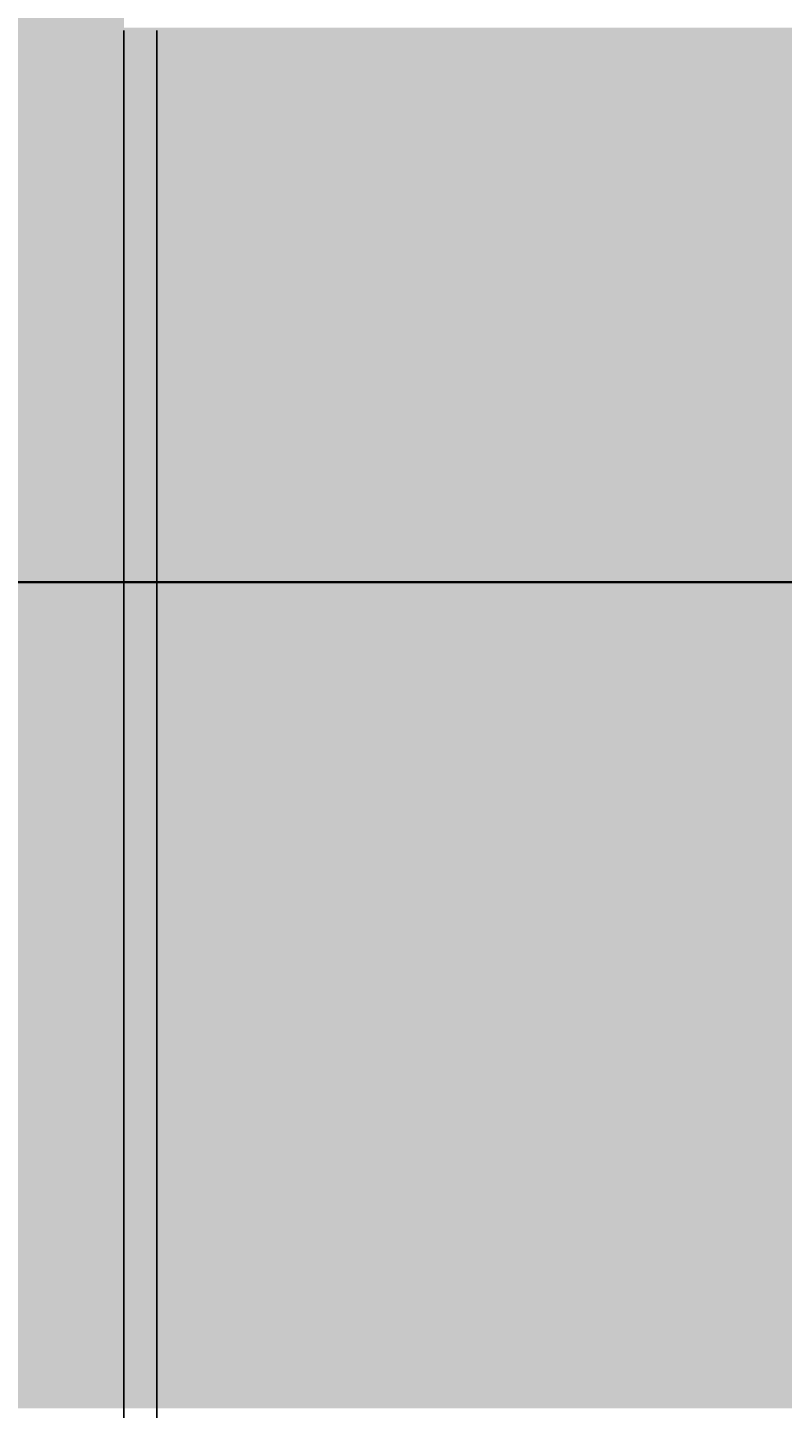
# Model space of a CAD drawing. Units: feet. Extents: x 2695 to 2912, y 795 to 1139.
# Tile 29 of 83: x 2808 to 2825, y 906 to 937. Entities that reach past the tile are written whole.
import ezdxf

# ---------------------------------------------------------------- set-up
doc = ezdxf.new("R2010")
doc.units = ezdxf.units.FT
for name, color, linetype, lineweight in [('A-ANNO-DIMS', 2, 'Continuous', 18), ('A-ELEV', 7, 'Continuous', 35), ('A-ELEV-PATT', 252, 'Continuous', 13)]:
    doc.layers.add(name, color=color, linetype=linetype, lineweight=lineweight)
doc.styles.get("Standard").update_dxf_attribs({"font": 'arial.ttf'})
doc.dimstyles.get("Standard").update_dxf_attribs({"dimtxt": 0.18, "dimasz": 0.18, "dimexe": 0.18, "dimexo": 0.0625, "dimgap": 0.09, "dimtad": 0, "dimtih": 1, "dimtoh": 1, "dimdec": 1, "dimzin": 0, "dimdsep": 46, "dimlunit": 3, "dimtxsty": 'Standard', "dimcen": 0.09, "dimadec": 0, "dimazin": 0, "dimtfac": 1, "dimtdec": 1, "dimtofl": 0, "dimtmove": 0, "dimatfit": 3, "dimfxl": 1, "dimtolj": 1, "dimtzin": 0, "dimarcsym": 0})

# ---------------------------------------------------------------- blocks, each defined once
blk = doc.blocks.new('*D14')
at = {"layer": 'A-ANNO-DIMS', "color": 0, "lineweight": -2, "transparency": 16777216}
for p, q in [((2838.439, 905.514), (2911.424, 905.514)), ((2911.244, 905.334), (2911.244, 890.368)), ((2911.244, 875.037), (2911.244, 890.004)), ((2758.214, 874.857), (2911.424, 874.857))]:
    blk.add_line(p, q, dxfattribs=at)
at = {"layer": 'A-ANNO-DIMS', "color": 0, "transparency": 16777216}
for points in [[(2911.214, 905.334), (2911.274, 905.334), (2911.244, 905.514)], [(2911.214, 875.037), (2911.274, 875.037), (2911.244, 874.857)]]:
    blk.add_solid(points, dxfattribs=at)
at = {"layer": 'Defpoints', "color": 0, "transparency": 16777216}
for p in [(2838.377, 905.514), (2911.244, 905.514), (2758.151, 874.857)]:
    blk.add_point(p, dxfattribs=at)
at = {"layer": 'A-ANNO-DIMS', "color": 0, "transparency": 16777216, "insert": (2911.244, 890.186), "char_height": 0.18, "attachment_point": 5}
blk.add_mtext('\\A1;30.66', dxfattribs=at)
blk = doc.blocks.new('*D52')
at = {"layer": 'A-ANNO-DIMS', "color": 0, "lineweight": -2, "transparency": 16777216}
for p, q in [((2810.041, 936.868), (2810.041, 794.976)), ((2810.789, 936.868), (2810.789, 794.976)), ((2809.861, 795.156), (2809.681, 795.156)), ((2810.969, 795.156), (2811.149, 795.156))]:
    blk.add_line(p, q, dxfattribs=at)
at = {"layer": 'A-ANNO-DIMS', "color": 0, "transparency": 16777216}
for points in [[(2809.861, 795.186), (2809.861, 795.126), (2810.041, 795.156)], [(2810.969, 795.186), (2810.969, 795.126), (2810.789, 795.156)]]:
    blk.add_solid(points, dxfattribs=at)
at = {"layer": 'Defpoints', "color": 0, "transparency": 16777216}
for p in [(2810.041, 936.931), (2810.789, 936.931), (2810.789, 795.156)]:
    blk.add_point(p, dxfattribs=at)
at = {"layer": 'A-ANNO-DIMS', "color": 0, "transparency": 16777216, "insert": (2810.415, 795.156), "char_height": 0.18, "attachment_point": 5}
blk.add_mtext('\\A1;0.75', dxfattribs=at)

msp = doc.modelspace()

# ---------------------------------------------------------------- hatches: boundary and pattern name
at = {"layer": 'A-ELEV-PATT'}
h = msp.add_hatch(color=256, dxfattribs=at)
h.set_gradient(color1=(255, 255, 255), tint=1)
h.paths.add_polyline_path([(2770.6361, 1122.9306), (2710.6361, 1122.9306), (2710.6361, 1118.4096), (2770.6361, 1118.4096)])
h.paths.add_polyline_path([(2890.6361, 1107.8588), (2770.6361, 1107.8588), (2770.6361, 1103.3378), (2890.6361, 1103.3378)])
h.paths.add_polyline_path([(2890.6361, 1062.9306), (2710.6361, 1062.9306), (2710.6361, 1056.9306), (2710.6361, 936.9306), (2710.6361, 924.3105), (2716.5358, 924.3105), (2890.6361, 924.3105), (2890.6361, 936.9306), (2715.8852, 936.9306), (2715.8852, 1050.3105), (2890.6361, 1050.3105)])
h.paths.add_polyline_path([(2716.5358, 924.3105), (2710.6361, 924.3105), (2710.6361, 810.9306), (2716.5358, 810.9306)])
h = msp.add_hatch(color=256, dxfattribs=at)
h.set_gradient(color1=(147, 149, 152), color2=(147, 149, 152), tint=1)
h.paths.add_polyline_path([(2770.6361, 1118.4096), (2710.6361, 1118.4096), (2710.6361, 1062.9306), (2770.6361, 1062.9306)])
h.paths.add_polyline_path([(2890.6361, 1103.3378), (2770.6361, 1103.3378), (2770.6361, 1062.9306), (2890.6361, 1062.9306)])
h.paths.add_polyline_path([(2730.7081, 1048.1052), (2755.1125, 1048.1052), (2755.1125, 936.9306), (2770.6361, 936.9306), (2770.6361, 1050.3105), (2715.8852, 1050.3105), (2715.8852, 936.9306), (2730.7081, 936.9306)])
h.paths.add_polyline_path([(2890.6361, 1050.3105), (2770.6361, 1050.3105), (2770.6361, 971.9673), (2778.0341, 971.9673), (2778.0341, 1020.8235), (2843.575, 1020.8235), (2843.575, 971.9673), (2890.6361, 971.9673)])
h.paths.add_polyline_path([(2888.1882, 970.7156), (2843.575, 970.7156), (2843.575, 964.8267), (2888.1882, 964.8267)])
h.paths.add_polyline_path([(2888.1882, 964.1328), (2843.575, 964.1328), (2843.575, 956.614), (2888.1882, 956.614)])
h.paths.add_polyline_path([(2888.1882, 955.9202), (2843.575, 955.9202), (2843.575, 949.2892), (2888.1882, 949.2892)])
h.paths.add_polyline_path([(2888.1882, 948.5954), (2843.575, 948.5954), (2843.575, 941.3507), (2888.1882, 941.3507)])
h.paths.add_polyline_path([(2888.1882, 940.6569), (2843.575, 940.6569), (2843.575, 936.9306), (2888.1882, 936.9306)])
h.paths.add_polyline_path([(2890.6361, 970.7156), (2888.9368, 970.7156), (2888.9368, 964.8267), (2890.6361, 964.8267)])
h.paths.add_polyline_path([(2890.6361, 964.1328), (2888.9368, 964.1328), (2888.9368, 956.614), (2890.6361, 956.614)])
h.paths.add_polyline_path([(2890.6361, 955.9202), (2888.9368, 955.9202), (2888.9368, 949.2892), (2890.6361, 949.2892)])
h.paths.add_polyline_path([(2890.6361, 940.6569), (2888.9368, 940.6569), (2888.9368, 936.9306), (2890.6361, 936.9306)])
h.paths.add_polyline_path([(2890.6361, 948.5954), (2888.9368, 948.5954), (2888.9368, 941.3507), (2890.6361, 941.3507)])
h.paths.add_polyline_path([(2772.5216, 970.7156), (2770.6361, 970.7156), (2770.6361, 964.8267), (2772.5216, 964.8267)])
h.paths.add_polyline_path([(2772.5216, 964.1328), (2770.6361, 964.1328), (2770.6361, 956.614), (2772.5216, 956.614)])
h.paths.add_polyline_path([(2772.5216, 955.9202), (2770.6361, 955.9202), (2770.6361, 949.2892), (2772.5216, 949.2892)])
h.paths.add_polyline_path([(2772.5216, 948.5954), (2770.6361, 948.5954), (2770.6361, 941.3507), (2772.5216, 941.3507)])
h.paths.add_polyline_path([(2772.5216, 940.6569), (2770.6361, 940.6569), (2770.6361, 936.9306), (2772.5216, 936.9306)])
h.paths.add_polyline_path([(2778.0341, 940.6569), (2773.2702, 940.6569), (2773.2702, 936.9306), (2778.0341, 936.9306)])
h.paths.add_polyline_path([(2778.0341, 970.7156), (2773.2702, 970.7156), (2773.2702, 964.8267), (2778.0341, 964.8267)])
h.paths.add_polyline_path([(2778.0341, 964.1328), (2773.2702, 964.1328), (2773.2702, 956.614), (2778.0341, 956.614)])
h.paths.add_polyline_path([(2778.0341, 955.9202), (2773.2702, 955.9202), (2773.2702, 949.2892), (2778.0341, 949.2892)])
h.paths.add_polyline_path([(2778.0341, 948.5954), (2773.2702, 948.5954), (2773.2702, 941.3507), (2778.0341, 941.3507)])
h.paths.add_polyline_path([(2810.0407, 940.6569), (2780.0341, 940.6569), (2780.0341, 936.9306), (2810.0407, 936.9306)])
h.paths.add_polyline_path([(2890.6361, 924.3105), (2770.6361, 924.3105), (2770.6361, 810.9306), (2773.5029, 810.9306), (2773.5029, 905.5143), (2805.9398, 905.5143), (2838.3767, 905.5143), (2838.3767, 810.9306), (2890.6361, 810.9306)])

# ---------------------------------------------------------------- linework, layer by layer
at = {"layer": 'A-ELEV'}
msp.add_lwpolyline([(2890.6361, 936.9306), (2890.6361, 924.3105), (2710.6361, 924.3105), (2710.6361, 936.9306)], dxfattribs=at)

# ---------------------------------------------------------------- dimensions: what is measured, and where the dimension line sits
at = {"layer": 'A-ANNO-DIMS'}
dim = msp.add_linear_dim(base=(2810.7893, 795.1556), p1=(2810.0407, 936.9306), p2=(2810.7893, 936.9306), dimstyle='Standard', override={"dimdec": 2, "dimlfac": 1, "dimrnd": 0, "dimzin": 0, "dimdsep": 46, "dimlunit": 2}, dxfattribs=at)
dim.commit()
dim.dimension.update_dxf_attribs({"geometry": '*D52', "text_midpoint": (2810.415, 795.1556)})
dim = msp.add_linear_dim(base=(2911.2444, 905.5143), p1=(2758.1515, 874.8571), p2=(2838.3767, 905.5143), angle=90, dimstyle='Standard', override={"dimdec": 2, "dimlfac": 1, "dimrnd": 0, "dimzin": 0, "dimdsep": 46, "dimlunit": 2}, dxfattribs=at)
dim.commit()
dim.dimension.update_dxf_attribs({"geometry": '*D14', "text_midpoint": (2911.2444, 890.1857)})

doc.saveas('drawing.dxf')
